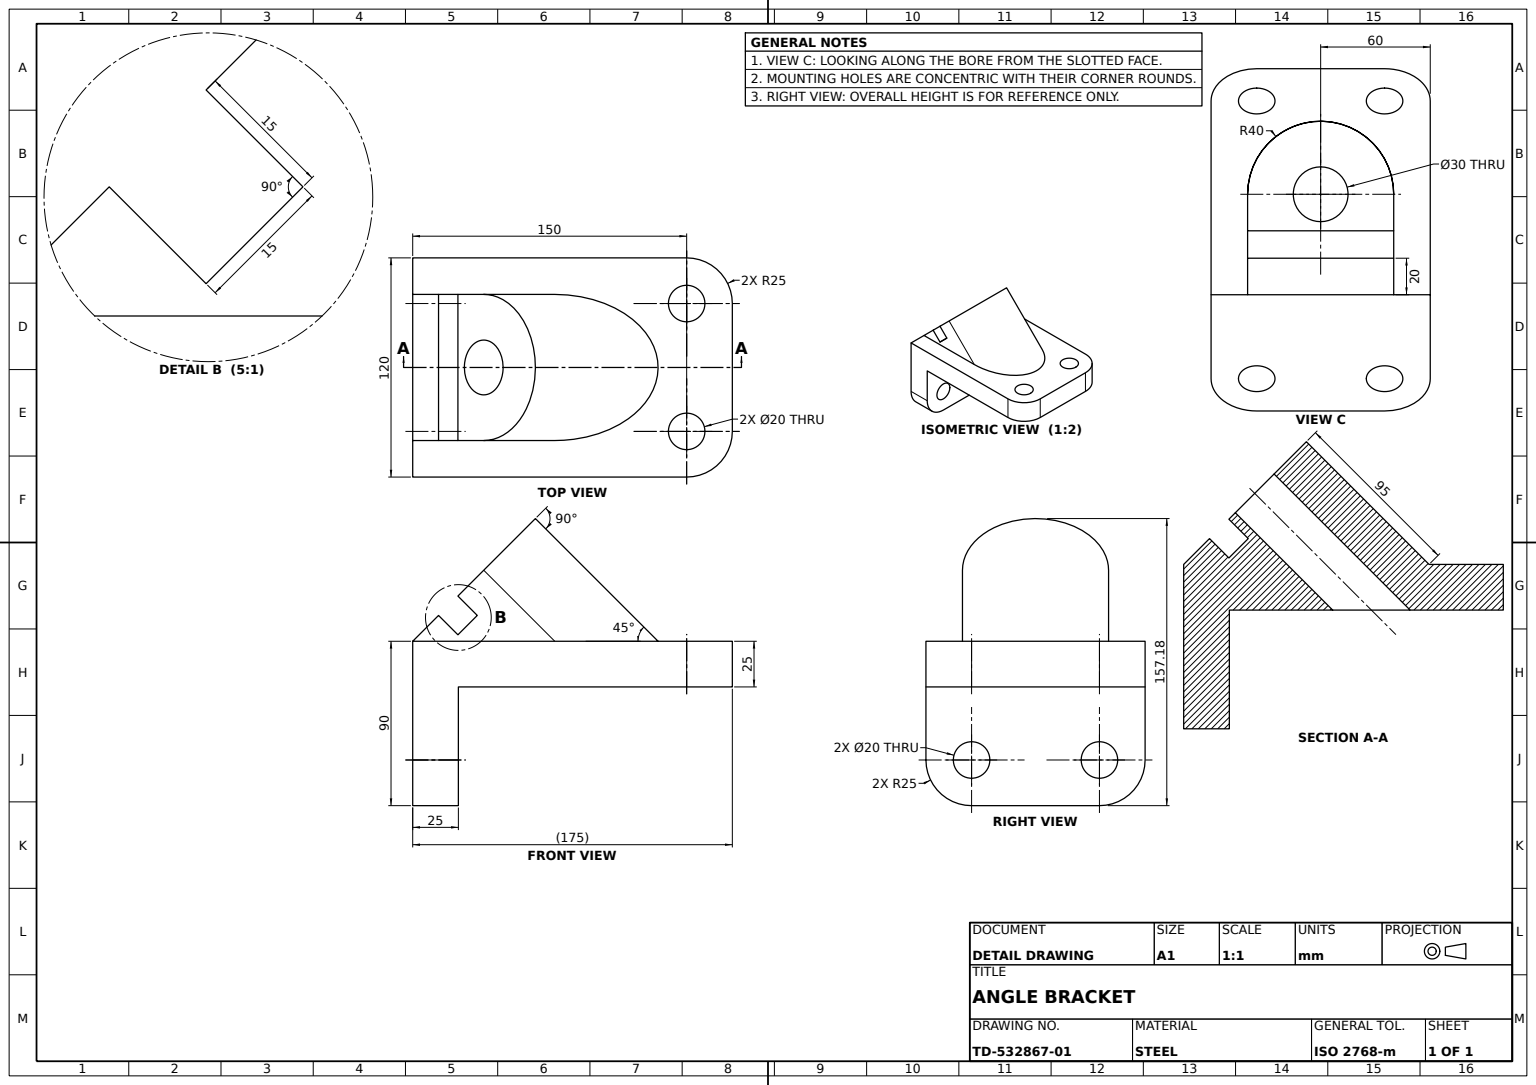
SolidWorks part; units mm, degrees
material "Plain Carbon Steel"
ref_plane "Front Plane" through (0, 0, 0) normal (0, 0, 1) x (1, 0, 0)
ref_plane "Top Plane" through (0, 0, 0) normal (0, 1, 0) x (1, 0, 0)
ref_plane "Right Plane" through (0, 0, 0) normal (1, 0, 0) x (0, 0, -1)
sketch "Upright Plate Sketch" plane through (0, 0, 0) normal (0, 0, 1) x (1, 0, 0)
  line L1 (-60, 45) -> (60, 45)
  line L2 (-60, 45) -> (-60, -20)
  line L3 (-35, -45) -> (35, -45)
  line L4 (60, 45) -> (60, -20)
  line L5 (-60, 45) -> (60, -45) construction
  line L6 (-60, -45) -> (60, 45) construction
  arc A0 (60, -20) -> (35, -45) centre (35, -20) cw
  arc A1 (-35, -45) -> (-60, -20) centre (-35, -20) cw
  circle A2 centre (-35, -20) radius 10
  circle A3 centre (35, -20) radius 10
  point P0 (0, 0)
  dimension "D3" = 25
  dimension "D4" = 20
  dimension "D5" = 20
  dimension "D1" = 90
  dimension "D2" = 120
extrude "Upright Plate" add sketch "Upright Plate Sketch" against normal blind 25
sketch "Base Plate Sketch" plane through (60, 0, 0) normal (1, 0, 0) x (0, 0, -1)
  line L0 (25, 45) -> (175, 45)
  line L1 (175, 45) -> (175, 20)
  line L2 (175, 20) -> (25, 20)
  line L3 (25, -20) -> (25, 45) construction
  line L4 (25, 20) -> (25, 45)
  dimension "D1" = 150
  dimension "D2" = 25
extrude "Base Plate" add sketch "Base Plate Sketch" against normal blind 120
fillet "Base Plate Corner Fillets R25" radius 25 2 edges at (-60, 32.5, -175) (60, 32.5, -175)
sketch "Base Plate Holes Sketch" plane through (0, 45, 0) normal (0, 1, 0) x (1, 0, 0)
  circle A0 centre (35, 150) radius 10
  circle A1 centre (-35, 150) radius 10
  dimension "D1" = 20
  dimension "D2" = 20
extrude "Base Plate Holes" cut sketch "Base Plate Holes Sketch" against normal through all
sketch "Wedge Support Sketch" plane through (0, 0, 0) normal (1, 0, 0) x (0, 0, -1)
  line L0 (134.3503, 45) -> (67.1751, 112.1751)
  line L1 (150, 45) -> (0, 45) construction
  line L2 (67.1751, 112.1751) -> (0, 45)
  line L3 (0, 45) -> (134.3503, 45)
  dimension "D1" = 45
  dimension "D2" = 95
extrude "Wedge Support" add sketch "Wedge Support Sketch" along normal mid plane 120 contours L2 L3 L0
sketch "Lug Profile Sketch" plane through (0, 22.5, 22.5) normal (0, 0.7071, 0.7071) x (1, 0, 0)
  line L0 (-40, 86.8198) -> (-40, 31.8198)
  line L1 (60, 31.8198) -> (-60, 31.8198) construction
  line L2 (-40, 31.8198) -> (40, 31.8198)
  line L3 (40, 31.8198) -> (40, 86.8198)
  line L4 (0, 0) -> (0, 51.1015) construction
  line L5 (60, 126.8198) -> (-60, 126.8198) construction
  arc A0 (40, 86.8198) -> (-40, 86.8198) centre (0, 86.8198) ccw
  circle A1 centre (0, 86.8198) radius 15
  line M6 (-60, 126.8198) -> (-60, 31.8198)
  line M7 (-60, 31.8198) -> (60, 31.8198)
  line M8 (60, 31.8198) -> (60, 126.8198)
  line M9 (60, 126.8198) -> (-60, 126.8198)
  dimension "D1" = 40
  dimension "D2" = 30
extrude "Lug Profile Cut" cut sketch "Lug Profile Sketch" against normal up to surface (55 mm away) contours A0 L0 M9 M6 M7 | A0 L3 M7 M8 M9 | A1
sketch "Lug Bore Sketch" plane through (0, 22.5, 22.5) normal (0, 0.7071, 0.7071) x (1, 0, 0)
  circle A0 centre (0, 86.8198) radius 15 construction
  circle A1 centre (0, 86.8198) radius 15
extrude "Lug Bore" cut sketch "Lug Bore Sketch" against normal through all
sketch "Lug Slot Sketch" plane through (0, 22.5, 22.5) normal (0, 0.7071, 0.7071) x (1, 0, 0)
  line L0 (-40, 66.8198) -> (40, 66.8198)
  line L1 (-40, 31.8198) -> (-40, 86.8198) construction
  line L2 (40, 31.8198) -> (40, 86.8198) construction
  line L3 (40, 66.8198) -> (40, 51.8198)
  line L4 (40, 86.8198) -> (40, 31.8198) construction
  line L5 (40, 51.8198) -> (-40, 51.8198)
  line L6 (-40, 51.8198) -> (-40, 66.8198)
  line L7 (40, 31.8198) -> (-40, 31.8198) construction
  dimension "D1" = 15
  dimension "D2" = 20
extrude "Lug Slot 15x20" cut sketch "Lug Slot Sketch" against normal blind 15
